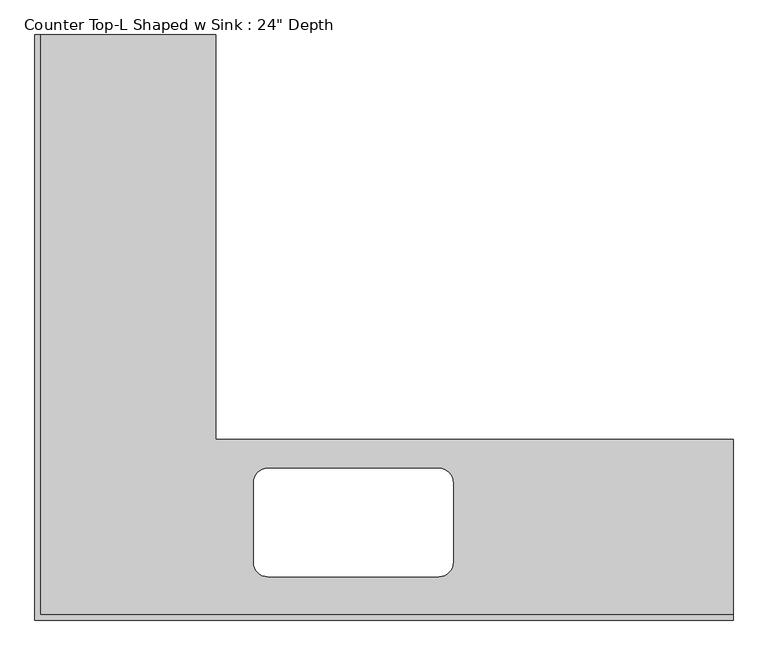
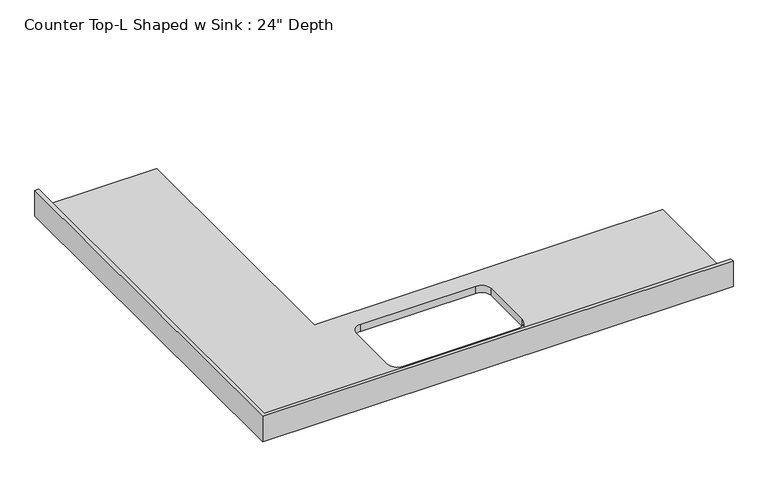
"""IFC4 building model written with IfcOpenShell, lengths in millimetres: furniture geometry."""

from ifc_helpers import new_model, si_unit, frame, origin, place, context, project, spatial, polyline, circle_curve, source, transform, mapped, element, save
from ifc_brep_helpers import plane_surface, revolved_surface, advanced_brep


def furniture_aa189fe6(model_context):
    return source(origin(), model_context, "Body", "AdvancedBrep", [
        advanced_brep(
        [(-565.4622951, 2057.4, 914.4), (-1181.4122951, 2057.4, 914.4), (-1181.4122951, 19.05, 914.4), (1252.3702343, 19.05, 914.4), (1252.3702343, 635.0, 914.4), (-565.4622951, 635.0, 914.4), (218.381846, 152.4, 914.4), (-381.7128423, 152.4, 914.4), (-432.5128423, 203.2, 914.4), (-432.5128423, 482.6, 914.4), (-381.7128423, 533.4, 914.4), (218.381846, 533.4, 914.4), (269.181846, 482.6, 914.4), (269.181846, 203.2, 914.4), (1252.3702343, 0.0, 876.3), (-1200.4622951, 0.0, 876.3), (-1200.4622951, 2057.4, 876.3), (-565.4622951, 2057.4, 876.3), (-565.4622951, 635.0, 876.3), (1252.3702343, 635.0, 876.3), (218.381846, 152.4, 876.3), (269.181846, 203.2, 876.3), (269.181846, 482.6, 876.3), (218.381846, 533.4, 876.3), (-381.7128423, 533.4, 876.3), (-432.5128423, 482.6, 876.3), (-432.5128423, 203.2, 876.3), (-381.7128423, 152.4, 876.3), (1252.3702343, 0.0, 1016.0), (-1200.4622951, 0.0, 1016.0), (-1200.4622951, 2057.4, 1016.0), (-1181.4122951, 2057.4, 1016.0), (1252.3702343, 19.05, 1016.0), (-1181.4122951, 19.05, 1016.0)],
        [
            (0, 1),
            (1, 2),
            (2, 3),
            (3, 4),
            (4, 5),
            (5, 0),
            (6, 7),
            (7, 8, circle_curve(frame((-381.7128423, 203.2, 914.4), z_axis=(0.0, 0.0, -1.0), x_axis=(1.0, 0.0, 0.0)), 50.8)),
            (8, 9),
            (9, 10, circle_curve(frame((-381.7128423, 482.6, 914.4), z_axis=(0.0, 0.0, -1.0), x_axis=(1.0, 0.0, 0.0)), 50.8)),
            (10, 11),
            (11, 12, circle_curve(frame((218.381846, 482.6, 914.4), z_axis=(0.0, 0.0, -1.0), x_axis=(1.0, 0.0, 0.0)), 50.8)),
            (12, 13),
            (13, 6, circle_curve(frame((218.381846, 203.2, 914.4), z_axis=(0.0, 0.0, -1.0), x_axis=(1.0, 0.0, 0.0)), 50.8)),
            (14, 15),
            (15, 16),
            (16, 17),
            (17, 18),
            (18, 19),
            (19, 14),
            (20, 21, circle_curve(frame((218.381846, 203.2, 876.3), z_axis=(0.0, 0.0, 1.0), x_axis=(1.0, 0.0, 0.0)), 50.8)),
            (21, 22),
            (22, 23, circle_curve(frame((218.381846, 482.6, 876.3), z_axis=(0.0, 0.0, 1.0), x_axis=(1.0, 0.0, 0.0)), 50.8)),
            (23, 24),
            (24, 25, circle_curve(frame((-381.7128423, 482.6, 876.3), z_axis=(0.0, 0.0, 1.0), x_axis=(1.0, 0.0, 0.0)), 50.8)),
            (25, 26),
            (26, 27, circle_curve(frame((-381.7128423, 203.2, 876.3), z_axis=(0.0, 0.0, 1.0), x_axis=(1.0, 0.0, 0.0)), 50.8)),
            (27, 20),
            (14, 28),
            (28, 29),
            (29, 15),
            (29, 30),
            (30, 16),
            (30, 31),
            (31, 1),
            (0, 17),
            (5, 18),
            (4, 19),
            (3, 32),
            (32, 28),
            (13, 21),
            (20, 6),
            (12, 22),
            (11, 23),
            (10, 24),
            (9, 25),
            (8, 26),
            (7, 27),
            (32, 33),
            (33, 31),
            (2, 33),
        ],
        [
            plane_surface(frame((-1200.4622951, 0.0, 914.4), z_axis=(0.0, 0.0, 1.0), x_axis=(-1.0, 0.0, 0.0))),
            plane_surface(frame((-1200.4622951, 0.0, 876.3), z_axis=(0.0, 0.0, -1.0), x_axis=(1.0, 0.0, 0.0))),
            plane_surface(frame((1252.3702343, 0.0, 914.4), z_axis=(0.0, -1.0, 0.0), x_axis=(0.0, 0.0, -1.0))),
            plane_surface(frame((-1200.4622951, 0.0, 914.4), z_axis=(-1.0, 0.0, 0.0), x_axis=(0.0, 0.0, -1.0))),
            plane_surface(frame((-1200.4622951, 2057.4, 914.4), z_axis=(0.0, 1.0, 0.0), x_axis=(0.0, 0.0, -1.0))),
            plane_surface(frame((-565.4622951, 2057.4, 914.4), z_axis=(1.0, 0.0, 0.0), x_axis=(0.0, 0.0, -1.0))),
            plane_surface(frame((-565.4622951, 635.0, 914.4), z_axis=(0.0, 1.0, 0.0), x_axis=(0.0, 0.0, -1.0))),
            plane_surface(frame((1252.3702343, 635.0, 914.4), z_axis=(1.0, 0.0, 0.0), x_axis=(0.0, 0.0, -1.0))),
            revolved_surface(polyline([(269.181846, 203.2, 876.3), (269.181846, 203.2, 914.4)]), (218.381846, 203.2, 0.0), (0.0, 0.0, -1.0)),
            plane_surface(frame((269.181846, 203.2, 914.4), z_axis=(-1.0, 0.0, 0.0), x_axis=(0.0, 0.0, -1.0))),
            revolved_surface(polyline([(269.181846, 482.6, 876.3), (269.181846, 482.6, 914.4)]), (218.381846, 482.6, 0.0), (0.0, 0.0, -1.0)),
            plane_surface(frame((218.381846, 533.4, 914.4), z_axis=(0.0, -1.0, 0.0), x_axis=(0.0, 0.0, -1.0))),
            revolved_surface(polyline([(-330.91284229999997, 482.6, 876.3), (-330.91284229999997, 482.6, 914.4)]), (-381.7128423, 482.6, 0.0), (0.0, 0.0, -1.0)),
            plane_surface(frame((-432.5128423, 482.6, 914.4), z_axis=(1.0, 0.0, 0.0), x_axis=(0.0, 0.0, -1.0))),
            revolved_surface(polyline([(-330.91284229999997, 203.2, 876.3), (-330.91284229999997, 203.2, 914.4)]), (-381.7128423, 203.2, 0.0), (0.0, 0.0, -1.0)),
            plane_surface(frame((-381.7128423, 152.4, 914.4), z_axis=(0.0, 1.0, 0.0), x_axis=(0.0, 0.0, -1.0))),
            plane_surface(frame((-1200.4622951, 0.0, 1016.0), z_axis=(0.0, 0.0, 1.0), x_axis=(0.0, 1.0, 0.0))),
            plane_surface(frame((-1200.4622951, 19.05, 1016.0), z_axis=(0.0, 1.0, 0.0), x_axis=(0.0, 0.0, -1.0))),
            plane_surface(frame((-1181.4122951, 2057.4, 1016.0), z_axis=(1.0, 0.0, 0.0), x_axis=(0.0, 0.0, -1.0))),
        ],
        [
            (0, [[1, 2, 3, 4, 5, 6], [7, 8, 9, 10, 11, 12, 13, 14]]),
            (1, [[15, 16, 17, 18, 19, 20], [21, 22, 23, 24, 25, 26, 27, 28]]),
            (2, [[29, 30, 31, -15]]),
            (3, [[-31, 32, 33, -16]]),
            (4, [[34, 35, -1, 36, -17, -33]]),
            (5, [[37, -18, -36, -6]]),
            (6, [[38, -19, -37, -5]]),
            (7, [[-38, -4, 39, 40, -29, -20]]),
            (8, [[41, -21, 42, -14]]),
            (9, [[43, -22, -41, -13]]),
            (10, [[44, -23, -43, -12]]),
            (11, [[45, -24, -44, -11]]),
            (12, [[46, -25, -45, -10]]),
            (13, [[47, -26, -46, -9]]),
            (14, [[48, -27, -47, -8]]),
            (15, [[-42, -28, -48, -7]]),
            (16, [[-30, -40, 49, 50, -34, -32]]),
            (17, [[-3, 51, -49, -39]]),
            (18, [[-51, -2, -35, -50]]),
        ],
    ),
    ])


if __name__ == "__main__":
    model = new_model("IFC4")
    model_context = context("Model", 3, world=origin())
    ifc_project = project(units=[si_unit("LENGTHUNIT", "METRE", prefix="MILLI")], contexts=[model_context])
    site = spatial("IfcSite", under=ifc_project)
    building = spatial("IfcBuilding", under=site)
    placement = place(None, origin())
    furniture_shape = furniture_aa189fe6(model_context)
    element("IfcFurniture", 1, ObjectType="Counter Top-L Shaped w Sink : 24\" Depth", at=placement, inside=building, context=model_context, shape_type="MappedRepresentation", body=[
        mapped(furniture_shape, transform((0.0, 0.0, 0.0), x_axis=(1.0, 0.0, 0.0), y_axis=(0.0, 1.0, 0.0), z_axis=(0.0, 0.0, 1.0))),
    ])
    save(model, "model.ifc")

# Revit data of these elements
# Type "Counter Top-L Shaped w Sink : 24\" Depth"
#   Assembly Code = "C1030400"
#   Counter Thickness = 0' - 1 1/2"
#   Depth = 2' - 1"
#   Height = 3' - 0"
#   Length - Leg 1 [instance default] = 8' - 0"
#   Length - Leg 2 [instance default] = 6' - 0"
#   Sink Location [instance default] = 3' - 0"
#   Sink Location To Wall [instance default] = 0' - 6"
#   Sink Opening Depth [instance default] = 1' - 3"
#   Sink Opening Width [instance default] = 3' - 3"
#   Counter Top Material = none
#   Default Elevation = 0
# Element 1 (IfcFurniture, "Counter Top-L Shaped w Sink : 24\" Depth")
#   Length - Leg 1 = 8' - 0.56821"
#   Length - Leg 2 = 6' - 9"
#   Sink Location = 2' - 6.23423"
#   Sink Opening Width = 2' - 3.62578"
#   Materials on its faces: "Counter Top"
# Materials
#   "Counter Top": class "Wood", colour RGB 226 177 128, transparency 0
